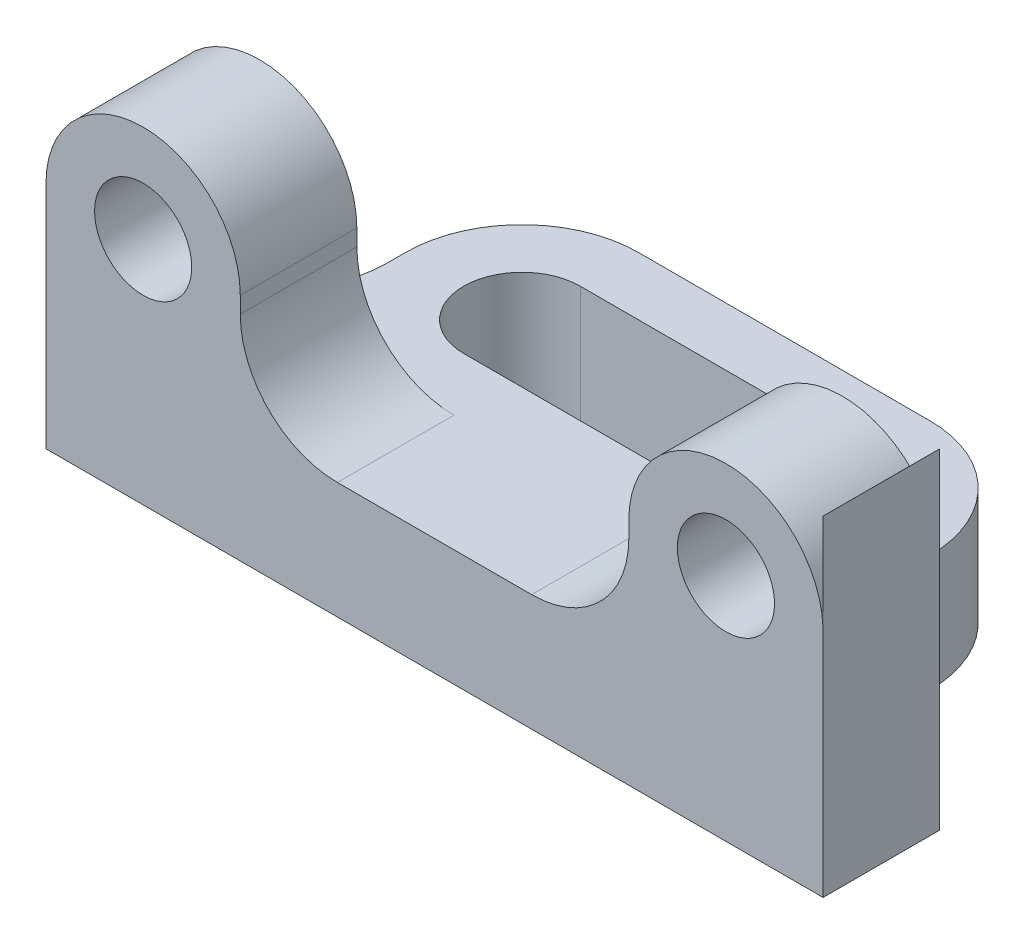
ISO-10303-21;
HEADER;
FILE_DESCRIPTION(('STEP AP214'),'2;1');
FILE_NAME('part.step','',(''),(''),'','','');
FILE_SCHEMA(('AUTOMOTIVE_DESIGN { 1 0 10303 214 1 1 1 1 }'));
ENDSEC;
DATA;
#1=APPLICATION_CONTEXT('core data for automotive mechanical design processes');
#2=APPLICATION_PROTOCOL_DEFINITION('international standard','automotive_design',2000,#1);
#3=PRODUCT_CONTEXT('',#1,'mechanical');
#4=PRODUCT('Part','Part','',(#3));
#5=PRODUCT_RELATED_PRODUCT_CATEGORY('part','',(#4));
#6=PRODUCT_DEFINITION_FORMATION('','',#4);
#7=PRODUCT_DEFINITION_CONTEXT('part definition',#1,'design');
#8=PRODUCT_DEFINITION('design','',#6,#7);
#9=PRODUCT_DEFINITION_SHAPE('','',#8);
#10=(LENGTH_UNIT() NAMED_UNIT(*) SI_UNIT(.MILLI.,.METRE.));
#11=(NAMED_UNIT(*) PLANE_ANGLE_UNIT() SI_UNIT($,.RADIAN.));
#12=(NAMED_UNIT(*) SI_UNIT($,.STERADIAN.) SOLID_ANGLE_UNIT());
#13=UNCERTAINTY_MEASURE_WITH_UNIT(LENGTH_MEASURE(1.E-05),#10,'distance_accuracy_value','');
#14=(GEOMETRIC_REPRESENTATION_CONTEXT(3) GLOBAL_UNCERTAINTY_ASSIGNED_CONTEXT((#13)) GLOBAL_UNIT_ASSIGNED_CONTEXT((#10,
#11,#12)) REPRESENTATION_CONTEXT('',''));
#15=CARTESIAN_POINT('',(0.,0.,0.));
#16=DIRECTION('',(0.,0.,1.));
#17=DIRECTION('',(1.,0.,0.));
#18=AXIS2_PLACEMENT_3D('',#15,#16,#17);
#19=CARTESIAN_POINT('',(0.,6.,0.));
#20=DIRECTION('',(0.,0.,-1.));
#21=DIRECTION('',(-1.,0.,0.));
#22=AXIS2_PLACEMENT_3D('',#19,#20,#21);
#23=PLANE('',#22);
#24=CARTESIAN_POINT('',(35.,11.844225053494,0.));
#25=DIRECTION('',(0.,0.,-1.));
#26=DIRECTION('',(-1.,0.,0.));
#27=AXIS2_PLACEMENT_3D('',#24,#25,#26);
#28=CIRCLE('',#27,2.5);
#29=CARTESIAN_POINT('',(32.5,11.844225053494,0.));
#30=VERTEX_POINT('',#29);
#31=EDGE_CURVE('E499',#30,#30,#28,.T.);
#32=ORIENTED_EDGE('',*,*,#31,.T.);
#33=EDGE_LOOP('',(#32));
#34=FACE_BOUND('',#33,.T.);
#35=CARTESIAN_POINT('',(5.,11.844225053494,0.));
#36=DIRECTION('',(0.,0.,-1.));
#37=DIRECTION('',(-1.,0.,0.));
#38=AXIS2_PLACEMENT_3D('',#35,#36,#37);
#39=CIRCLE('',#38,2.5);
#40=CARTESIAN_POINT('',(2.5,11.844225053494,0.));
#41=VERTEX_POINT('',#40);
#42=EDGE_CURVE('E505',#41,#41,#39,.T.);
#43=ORIENTED_EDGE('',*,*,#42,.T.);
#44=EDGE_LOOP('',(#43));
#45=FACE_BOUND('',#44,.T.);
#46=CARTESIAN_POINT('',(35.,11.844225053494,0.));
#47=DIRECTION('',(0.,0.,-1.));
#48=DIRECTION('',(-1.,0.,0.));
#49=AXIS2_PLACEMENT_3D('',#46,#47,#48);
#50=CIRCLE('',#49,5.);
#51=CARTESIAN_POINT('',(30.,11.844225053494,0.));
#52=VERTEX_POINT('',#51);
#53=CARTESIAN_POINT('',(39.9945012234225,12.0786552760139,0.));
#54=VERTEX_POINT('',#53);
#55=EDGE_CURVE('E467',#52,#54,#50,.T.);
#56=ORIENTED_EDGE('',*,*,#55,.F.);
#57=DIRECTION('',(0.,-1.,0.));
#58=VECTOR('',#57,1.);
#59=CARTESIAN_POINT('',(30.,17.,0.));
#60=LINE('',#59,#58);
#61=CARTESIAN_POINT('',(30.,11.,0.));
#62=VERTEX_POINT('',#61);
#63=EDGE_CURVE('E209',#52,#62,#60,.T.);
#64=ORIENTED_EDGE('',*,*,#63,.T.);
#65=CARTESIAN_POINT('',(25.,11.,0.));
#66=DIRECTION('',(0.,0.,-1.));
#67=DIRECTION('',(-1.,0.,0.));
#68=AXIS2_PLACEMENT_3D('',#65,#66,#67);
#69=CIRCLE('',#68,5.);
#70=CARTESIAN_POINT('',(25.,6.,0.));
#71=VERTEX_POINT('',#70);
#72=EDGE_CURVE('E47',#62,#71,#69,.T.);
#73=ORIENTED_EDGE('',*,*,#72,.T.);
#74=DIRECTION('',(1.,0.,0.));
#75=VECTOR('',#74,1.);
#76=CARTESIAN_POINT('',(0.,6.,0.));
#77=LINE('',#76,#75);
#78=CARTESIAN_POINT('',(15.,6.,0.));
#79=VERTEX_POINT('',#78);
#80=EDGE_CURVE('E259',#79,#71,#77,.T.);
#81=ORIENTED_EDGE('',*,*,#80,.F.);
#82=CARTESIAN_POINT('',(15.,11.,0.));
#83=DIRECTION('',(0.,0.,-1.));
#84=DIRECTION('',(-1.,0.,0.));
#85=AXIS2_PLACEMENT_3D('',#82,#83,#84);
#86=CIRCLE('',#85,5.);
#87=CARTESIAN_POINT('',(10.,11.,0.));
#88=VERTEX_POINT('',#87);
#89=EDGE_CURVE('E326',#79,#88,#86,.T.);
#90=ORIENTED_EDGE('',*,*,#89,.T.);
#91=DIRECTION('',(0.,-1.,0.));
#92=VECTOR('',#91,1.);
#93=CARTESIAN_POINT('',(10.,17.,0.));
#94=LINE('',#93,#92);
#95=CARTESIAN_POINT('',(10.,11.844225053494,0.));
#96=VERTEX_POINT('',#95);
#97=EDGE_CURVE('E493',#96,#88,#94,.T.);
#98=ORIENTED_EDGE('',*,*,#97,.F.);
#99=CARTESIAN_POINT('',(5.,11.844225053494,0.));
#100=DIRECTION('',(0.,0.,-1.));
#101=DIRECTION('',(-1.,0.,0.));
#102=AXIS2_PLACEMENT_3D('',#99,#100,#101);
#103=CIRCLE('',#102,5.);
#104=CARTESIAN_POINT('',(0.,11.844225053494,0.));
#105=VERTEX_POINT('',#104);
#106=EDGE_CURVE('E508',#105,#96,#103,.T.);
#107=ORIENTED_EDGE('',*,*,#106,.F.);
#108=DIRECTION('',(0.,-1.,0.));
#109=VECTOR('',#108,1.);
#110=CARTESIAN_POINT('',(0.,17.,0.));
#111=LINE('',#110,#109);
#112=CARTESIAN_POINT('',(0.,0.,0.));
#113=VERTEX_POINT('',#112);
#114=EDGE_CURVE('E487',#105,#113,#111,.T.);
#115=ORIENTED_EDGE('',*,*,#114,.T.);
#116=DIRECTION('',(1.,0.,0.));
#117=VECTOR('',#116,1.);
#118=CARTESIAN_POINT('',(0.,0.,0.));
#119=LINE('',#118,#117);
#120=CARTESIAN_POINT('',(40.,0.,0.));
#121=VERTEX_POINT('',#120);
#122=EDGE_CURVE('E227',#113,#121,#119,.T.);
#123=ORIENTED_EDGE('',*,*,#122,.T.);
#124=DIRECTION('',(0.,-1.,0.));
#125=VECTOR('',#124,1.);
#126=CARTESIAN_POINT('',(40.,17.,0.));
#127=LINE('',#126,#125);
#128=CARTESIAN_POINT('',(40.,17.,0.));
#129=VERTEX_POINT('',#128);
#130=EDGE_CURVE('E216',#129,#121,#127,.T.);
#131=ORIENTED_EDGE('',*,*,#130,.F.);
#132=DIRECTION('',(0.00111733143143493,0.999999375785041,0.));
#133=VECTOR('',#132,1.);
#134=CARTESIAN_POINT('',(39.9876594247451,5.95532050336561,0.));
#135=LINE('',#134,#133);
#136=EDGE_CURVE('E464',#54,#129,#135,.T.);
#137=ORIENTED_EDGE('',*,*,#136,.F.);
#138=EDGE_LOOP('',(#56,#64,#73,#81,#90,#98,#107,#115,#123,#131,#137));
#139=FACE_BOUND('',#138,.T.);
#140=ADVANCED_FACE('F41',(#34,#45,#139),#23,.F.);
#141=CARTESIAN_POINT('',(0.,17.,-6.));
#142=DIRECTION('',(0.,0.,1.));
#143=DIRECTION('',(1.,0.,0.));
#144=AXIS2_PLACEMENT_3D('',#141,#142,#143);
#145=PLANE('',#144);
#146=CARTESIAN_POINT('',(35.,11.844225053494,-6.));
#147=DIRECTION('',(0.,0.,-1.));
#148=DIRECTION('',(-1.,0.,0.));
#149=AXIS2_PLACEMENT_3D('',#146,#147,#148);
#150=CIRCLE('',#149,2.5);
#151=CARTESIAN_POINT('',(32.5,11.844225053494,-6.));
#152=VERTEX_POINT('',#151);
#153=EDGE_CURVE('E504',#152,#152,#150,.T.);
#154=ORIENTED_EDGE('',*,*,#153,.F.);
#155=EDGE_LOOP('',(#154));
#156=FACE_BOUND('',#155,.T.);
#157=CARTESIAN_POINT('',(35.,11.844225053494,-6.));
#158=DIRECTION('',(0.,0.,-1.));
#159=DIRECTION('',(-1.,0.,0.));
#160=AXIS2_PLACEMENT_3D('',#157,#158,#159);
#161=CIRCLE('',#160,5.);
#162=CARTESIAN_POINT('',(30.,11.844225053494,-6.));
#163=VERTEX_POINT('',#162);
#164=CARTESIAN_POINT('',(39.9945012234225,12.0786552760139,-5.99999999999999));
#165=VERTEX_POINT('',#164);
#166=EDGE_CURVE('E197',#163,#165,#161,.T.);
#167=ORIENTED_EDGE('',*,*,#166,.T.);
#168=DIRECTION('',(0.00111733143143494,0.999999375785041,0.));
#169=VECTOR('',#168,1.);
#170=CARTESIAN_POINT('',(39.9809554403412,-0.0446720060572272,-5.99999999999999));
#171=LINE('',#170,#169);
#172=CARTESIAN_POINT('',(40.,17.,-5.99999999999999));
#173=VERTEX_POINT('',#172);
#174=EDGE_CURVE('E203',#165,#173,#171,.T.);
#175=ORIENTED_EDGE('',*,*,#174,.T.);
#176=DIRECTION('',(0.,-1.,0.));
#177=VECTOR('',#176,1.);
#178=CARTESIAN_POINT('',(40.,17.,-6.));
#179=LINE('',#178,#177);
#180=CARTESIAN_POINT('',(40.,0.,-6.));
#181=VERTEX_POINT('',#180);
#182=EDGE_CURVE('E472',#173,#181,#179,.T.);
#183=ORIENTED_EDGE('',*,*,#182,.T.);
#184=DIRECTION('',(-1.,0.,0.));
#185=VECTOR('',#184,1.);
#186=CARTESIAN_POINT('',(0.,0.,-6.));
#187=LINE('',#186,#185);
#188=CARTESIAN_POINT('',(38.5,0.,-5.99999999999999));
#189=VERTEX_POINT('',#188);
#190=EDGE_CURVE('E479',#181,#189,#187,.T.);
#191=ORIENTED_EDGE('',*,*,#190,.T.);
#192=DIRECTION('',(0.,-1.,0.));
#193=VECTOR('',#192,1.);
#194=CARTESIAN_POINT('',(38.5,6.,-5.99999999999999));
#195=LINE('',#194,#193);
#196=CARTESIAN_POINT('',(38.5,6.,-5.99999999999999));
#197=VERTEX_POINT('',#196);
#198=EDGE_CURVE('E307',#197,#189,#195,.T.);
#199=ORIENTED_EDGE('',*,*,#198,.F.);
#200=DIRECTION('',(-1.,0.,0.));
#201=VECTOR('',#200,1.);
#202=CARTESIAN_POINT('',(0.,6.,-6.));
#203=LINE('',#202,#201);
#204=CARTESIAN_POINT('',(25.,6.,-6.));
#205=VERTEX_POINT('',#204);
#206=EDGE_CURVE('E232',#197,#205,#203,.T.);
#207=ORIENTED_EDGE('',*,*,#206,.T.);
#208=CARTESIAN_POINT('',(25.,11.,-6.));
#209=DIRECTION('',(0.,0.,1.));
#210=DIRECTION('',(1.,0.,0.));
#211=AXIS2_PLACEMENT_3D('',#208,#209,#210);
#212=CIRCLE('',#211,5.);
#213=CARTESIAN_POINT('',(30.,11.,-6.));
#214=VERTEX_POINT('',#213);
#215=EDGE_CURVE('E11',#205,#214,#212,.T.);
#216=ORIENTED_EDGE('',*,*,#215,.T.);
#217=DIRECTION('',(0.,-1.,0.));
#218=VECTOR('',#217,1.);
#219=CARTESIAN_POINT('',(30.,17.,-6.));
#220=LINE('',#219,#218);
#221=EDGE_CURVE('E61',#163,#214,#220,.T.);
#222=ORIENTED_EDGE('',*,*,#221,.F.);
#223=EDGE_LOOP('',(#167,#175,#183,#191,#199,#207,#216,#222));
#224=FACE_BOUND('',#223,.T.);
#225=ADVANCED_FACE('F212',(#156,#224),#145,.F.);
#226=CARTESIAN_POINT('',(0.,17.,-5.99999999999999));
#227=DIRECTION('',(0.,0.,-1.));
#228=DIRECTION('',(-1.,0.,0.));
#229=AXIS2_PLACEMENT_3D('',#226,#227,#228);
#230=PLANE('',#229);
#231=CARTESIAN_POINT('',(5.,11.844225053494,-6.));
#232=DIRECTION('',(0.,0.,-1.));
#233=DIRECTION('',(-1.,0.,0.));
#234=AXIS2_PLACEMENT_3D('',#231,#232,#233);
#235=CIRCLE('',#234,2.5);
#236=CARTESIAN_POINT('',(2.5,11.844225053494,-6.));
#237=VERTEX_POINT('',#236);
#238=EDGE_CURVE('E506',#237,#237,#235,.T.);
#239=ORIENTED_EDGE('',*,*,#238,.F.);
#240=EDGE_LOOP('',(#239));
#241=FACE_BOUND('',#240,.T.);
#242=DIRECTION('',(0.,-1.,0.));
#243=VECTOR('',#242,1.);
#244=CARTESIAN_POINT('',(0.,17.,-5.99999999999999));
#245=LINE('',#244,#243);
#246=CARTESIAN_POINT('',(0.,11.844225053494,-5.99999999999999));
#247=VERTEX_POINT('',#246);
#248=CARTESIAN_POINT('',(0.,0.,-5.99999999999999));
#249=VERTEX_POINT('',#248);
#250=EDGE_CURVE('E481',#247,#249,#245,.T.);
#251=ORIENTED_EDGE('',*,*,#250,.F.);
#252=CARTESIAN_POINT('',(5.,11.844225053494,-6.));
#253=DIRECTION('',(0.,0.,-1.));
#254=DIRECTION('',(-1.,0.,0.));
#255=AXIS2_PLACEMENT_3D('',#252,#253,#254);
#256=CIRCLE('',#255,5.);
#257=CARTESIAN_POINT('',(10.,11.844225053494,-6.));
#258=VERTEX_POINT('',#257);
#259=EDGE_CURVE('E57',#247,#258,#256,.T.);
#260=ORIENTED_EDGE('',*,*,#259,.T.);
#261=DIRECTION('',(0.,-1.,0.));
#262=VECTOR('',#261,1.);
#263=CARTESIAN_POINT('',(10.,17.,-6.));
#264=LINE('',#263,#262);
#265=CARTESIAN_POINT('',(10.,11.,-6.));
#266=VERTEX_POINT('',#265);
#267=EDGE_CURVE('E482',#258,#266,#264,.T.);
#268=ORIENTED_EDGE('',*,*,#267,.T.);
#269=CARTESIAN_POINT('',(15.,11.,-6.));
#270=DIRECTION('',(0.,0.,-1.));
#271=DIRECTION('',(-1.,0.,0.));
#272=AXIS2_PLACEMENT_3D('',#269,#270,#271);
#273=CIRCLE('',#272,5.);
#274=CARTESIAN_POINT('',(15.,6.,-6.));
#275=VERTEX_POINT('',#274);
#276=EDGE_CURVE('E334',#266,#275,#273,.F.);
#277=ORIENTED_EDGE('',*,*,#276,.T.);
#278=DIRECTION('',(1.,0.,0.));
#279=VECTOR('',#278,1.);
#280=CARTESIAN_POINT('',(0.,6.,-5.99999999999999));
#281=LINE('',#280,#279);
#282=CARTESIAN_POINT('',(1.49999999999996,6.,-5.99999999999999));
#283=VERTEX_POINT('',#282);
#284=EDGE_CURVE('E257',#283,#275,#281,.T.);
#285=ORIENTED_EDGE('',*,*,#284,.F.);
#286=DIRECTION('',(0.,-1.,0.));
#287=VECTOR('',#286,1.);
#288=CARTESIAN_POINT('',(1.49999999999996,6.,-5.99999999999999));
#289=LINE('',#288,#287);
#290=CARTESIAN_POINT('',(1.49999999999996,0.,-5.99999999999999));
#291=VERTEX_POINT('',#290);
#292=EDGE_CURVE('E292',#283,#291,#289,.T.);
#293=ORIENTED_EDGE('',*,*,#292,.T.);
#294=DIRECTION('',(1.,0.,0.));
#295=VECTOR('',#294,1.);
#296=CARTESIAN_POINT('',(0.,0.,-5.99999999999999));
#297=LINE('',#296,#295);
#298=EDGE_CURVE('E500',#249,#291,#297,.T.);
#299=ORIENTED_EDGE('',*,*,#298,.F.);
#300=EDGE_LOOP('',(#251,#260,#268,#277,#285,#293,#299));
#301=FACE_BOUND('',#300,.T.);
#302=ADVANCED_FACE('F365',(#241,#301),#230,.T.);
#303=CARTESIAN_POINT('',(38.5,6.,-11.));
#304=DIRECTION('',(0.,-1.,0.));
#305=DIRECTION('',(0.,0.,-1.));
#306=AXIS2_PLACEMENT_3D('',#303,#304,#305);
#307=CYLINDRICAL_SURFACE('',#306,5.);
#308=CARTESIAN_POINT('',(38.5,0.,-11.));
#309=DIRECTION('',(0.,1.,0.));
#310=DIRECTION('',(0.,0.,1.));
#311=AXIS2_PLACEMENT_3D('',#308,#309,#310);
#312=CIRCLE('',#311,5.);
#313=CARTESIAN_POINT('',(33.5,0.,-11.));
#314=VERTEX_POINT('',#313);
#315=EDGE_CURVE('E268',#189,#314,#312,.F.);
#316=ORIENTED_EDGE('',*,*,#315,.T.);
#317=DIRECTION('',(0.,-1.,0.));
#318=VECTOR('',#317,1.);
#319=CARTESIAN_POINT('',(33.5,6.,-11.));
#320=LINE('',#319,#318);
#321=CARTESIAN_POINT('',(33.5,6.,-11.));
#322=VERTEX_POINT('',#321);
#323=EDGE_CURVE('E306',#322,#314,#320,.T.);
#324=ORIENTED_EDGE('',*,*,#323,.F.);
#325=CARTESIAN_POINT('',(38.5,6.,-11.));
#326=DIRECTION('',(0.,1.,0.));
#327=DIRECTION('',(0.,0.,1.));
#328=AXIS2_PLACEMENT_3D('',#325,#326,#327);
#329=CIRCLE('',#328,5.);
#330=EDGE_CURVE('E240',#197,#322,#329,.F.);
#331=ORIENTED_EDGE('',*,*,#330,.F.);
#332=ORIENTED_EDGE('',*,*,#198,.T.);
#333=EDGE_LOOP('',(#316,#324,#331,#332));
#334=FACE_BOUND('',#333,.T.);
#335=ADVANCED_FACE('F393',(#334),#307,.F.);
#336=CARTESIAN_POINT('',(33.5,6.,0.));
#337=DIRECTION('',(-1.,0.,0.));
#338=DIRECTION('',(0.,0.,1.));
#339=AXIS2_PLACEMENT_3D('',#336,#337,#338);
#340=PLANE('',#339);
#341=DIRECTION('',(0.,0.,-1.));
#342=VECTOR('',#341,1.);
#343=CARTESIAN_POINT('',(33.5,0.,0.));
#344=LINE('',#343,#342);
#345=CARTESIAN_POINT('',(33.5,0.,-12.));
#346=VERTEX_POINT('',#345);
#347=EDGE_CURVE('E271',#314,#346,#344,.T.);
#348=ORIENTED_EDGE('',*,*,#347,.T.);
#349=DIRECTION('',(0.,-1.,0.));
#350=VECTOR('',#349,1.);
#351=CARTESIAN_POINT('',(33.5,6.,-12.));
#352=LINE('',#351,#350);
#353=CARTESIAN_POINT('',(33.5,6.,-12.));
#354=VERTEX_POINT('',#353);
#355=EDGE_CURVE('E302',#354,#346,#352,.T.);
#356=ORIENTED_EDGE('',*,*,#355,.F.);
#357=DIRECTION('',(0.,0.,-1.));
#358=VECTOR('',#357,1.);
#359=CARTESIAN_POINT('',(33.5,6.,0.));
#360=LINE('',#359,#358);
#361=EDGE_CURVE('E239',#322,#354,#360,.T.);
#362=ORIENTED_EDGE('',*,*,#361,.F.);
#363=ORIENTED_EDGE('',*,*,#323,.T.);
#364=EDGE_LOOP('',(#348,#356,#362,#363));
#365=FACE_BOUND('',#364,.T.);
#366=ADVANCED_FACE('F392',(#365),#340,.F.);
#367=CARTESIAN_POINT('',(27.5,6.,-12.));
#368=DIRECTION('',(0.,-1.,0.));
#369=DIRECTION('',(0.,0.,-1.));
#370=AXIS2_PLACEMENT_3D('',#367,#368,#369);
#371=CYLINDRICAL_SURFACE('',#370,6.);
#372=CARTESIAN_POINT('',(27.5,0.,-12.));
#373=DIRECTION('',(0.,1.,0.));
#374=DIRECTION('',(0.,0.,1.));
#375=AXIS2_PLACEMENT_3D('',#372,#373,#374);
#376=CIRCLE('',#375,6.);
#377=CARTESIAN_POINT('',(27.5,0.,-18.));
#378=VERTEX_POINT('',#377);
#379=EDGE_CURVE('E277',#378,#346,#376,.F.);
#380=ORIENTED_EDGE('',*,*,#379,.F.);
#381=DIRECTION('',(0.,-1.,0.));
#382=VECTOR('',#381,1.);
#383=CARTESIAN_POINT('',(27.5,6.,-18.));
#384=LINE('',#383,#382);
#385=CARTESIAN_POINT('',(27.5,6.,-18.));
#386=VERTEX_POINT('',#385);
#387=EDGE_CURVE('E305',#386,#378,#384,.T.);
#388=ORIENTED_EDGE('',*,*,#387,.F.);
#389=CARTESIAN_POINT('',(27.5,6.,-12.));
#390=DIRECTION('',(0.,1.,0.));
#391=DIRECTION('',(0.,0.,1.));
#392=AXIS2_PLACEMENT_3D('',#389,#390,#391);
#393=CIRCLE('',#392,6.);
#394=EDGE_CURVE('E245',#386,#354,#393,.F.);
#395=ORIENTED_EDGE('',*,*,#394,.T.);
#396=ORIENTED_EDGE('',*,*,#355,.T.);
#397=EDGE_LOOP('',(#380,#388,#395,#396));
#398=FACE_BOUND('',#397,.T.);
#399=ADVANCED_FACE('F390',(#398),#371,.T.);
#400=CARTESIAN_POINT('',(0.,6.,-18.));
#401=DIRECTION('',(0.,0.,-1.));
#402=DIRECTION('',(-1.,0.,0.));
#403=AXIS2_PLACEMENT_3D('',#400,#401,#402);
#404=PLANE('',#403);
#405=DIRECTION('',(1.,0.,0.));
#406=VECTOR('',#405,1.);
#407=CARTESIAN_POINT('',(0.,0.,-18.));
#408=LINE('',#407,#406);
#409=CARTESIAN_POINT('',(12.5,0.,-18.));
#410=VERTEX_POINT('',#409);
#411=EDGE_CURVE('E276',#410,#378,#408,.T.);
#412=ORIENTED_EDGE('',*,*,#411,.F.);
#413=DIRECTION('',(0.,-1.,0.));
#414=VECTOR('',#413,1.);
#415=CARTESIAN_POINT('',(12.5,6.,-18.));
#416=LINE('',#415,#414);
#417=CARTESIAN_POINT('',(12.5,6.,-18.));
#418=VERTEX_POINT('',#417);
#419=EDGE_CURVE('E297',#418,#410,#416,.T.);
#420=ORIENTED_EDGE('',*,*,#419,.F.);
#421=DIRECTION('',(1.,0.,0.));
#422=VECTOR('',#421,1.);
#423=CARTESIAN_POINT('',(0.,6.,-18.));
#424=LINE('',#423,#422);
#425=EDGE_CURVE('E244',#418,#386,#424,.T.);
#426=ORIENTED_EDGE('',*,*,#425,.T.);
#427=ORIENTED_EDGE('',*,*,#387,.T.);
#428=EDGE_LOOP('',(#412,#420,#426,#427));
#429=FACE_BOUND('',#428,.T.);
#430=ADVANCED_FACE('F384',(#429),#404,.T.);
#431=CARTESIAN_POINT('',(12.5,6.,-12.));
#432=DIRECTION('',(0.,-1.,0.));
#433=DIRECTION('',(0.,0.,-1.));
#434=AXIS2_PLACEMENT_3D('',#431,#432,#433);
#435=CYLINDRICAL_SURFACE('',#434,6.);
#436=CARTESIAN_POINT('',(12.5,0.,-12.));
#437=DIRECTION('',(0.,1.,0.));
#438=DIRECTION('',(0.,0.,1.));
#439=AXIS2_PLACEMENT_3D('',#436,#437,#438);
#440=CIRCLE('',#439,6.);
#441=CARTESIAN_POINT('',(6.5,0.,-12.));
#442=VERTEX_POINT('',#441);
#443=EDGE_CURVE('E284',#410,#442,#440,.T.);
#444=ORIENTED_EDGE('',*,*,#443,.T.);
#445=DIRECTION('',(0.,-1.,0.));
#446=VECTOR('',#445,1.);
#447=CARTESIAN_POINT('',(6.5,6.,-12.));
#448=LINE('',#447,#446);
#449=CARTESIAN_POINT('',(6.5,6.,-12.));
#450=VERTEX_POINT('',#449);
#451=EDGE_CURVE('E296',#450,#442,#448,.T.);
#452=ORIENTED_EDGE('',*,*,#451,.F.);
#453=CARTESIAN_POINT('',(12.5,6.,-12.));
#454=DIRECTION('',(0.,1.,0.));
#455=DIRECTION('',(0.,0.,1.));
#456=AXIS2_PLACEMENT_3D('',#453,#454,#455);
#457=CIRCLE('',#456,6.);
#458=EDGE_CURVE('E247',#418,#450,#457,.T.);
#459=ORIENTED_EDGE('',*,*,#458,.F.);
#460=ORIENTED_EDGE('',*,*,#419,.T.);
#461=EDGE_LOOP('',(#444,#452,#459,#460));
#462=FACE_BOUND('',#461,.T.);
#463=ADVANCED_FACE('F378',(#462),#435,.T.);
#464=CARTESIAN_POINT('',(6.5,6.,0.));
#465=DIRECTION('',(-1.,0.,0.));
#466=DIRECTION('',(0.,0.,1.));
#467=AXIS2_PLACEMENT_3D('',#464,#465,#466);
#468=PLANE('',#467);
#469=DIRECTION('',(0.,0.,-1.));
#470=VECTOR('',#469,1.);
#471=CARTESIAN_POINT('',(6.5,0.,0.));
#472=LINE('',#471,#470);
#473=CARTESIAN_POINT('',(6.5,0.,-11.));
#474=VERTEX_POINT('',#473);
#475=EDGE_CURVE('E283',#474,#442,#472,.T.);
#476=ORIENTED_EDGE('',*,*,#475,.F.);
#477=DIRECTION('',(0.,-1.,0.));
#478=VECTOR('',#477,1.);
#479=CARTESIAN_POINT('',(6.5,6.,-11.));
#480=LINE('',#479,#478);
#481=CARTESIAN_POINT('',(6.5,6.,-11.));
#482=VERTEX_POINT('',#481);
#483=EDGE_CURVE('E294',#482,#474,#480,.T.);
#484=ORIENTED_EDGE('',*,*,#483,.F.);
#485=DIRECTION('',(0.,0.,-1.));
#486=VECTOR('',#485,1.);
#487=CARTESIAN_POINT('',(6.5,6.,0.));
#488=LINE('',#487,#486);
#489=EDGE_CURVE('E249',#482,#450,#488,.T.);
#490=ORIENTED_EDGE('',*,*,#489,.T.);
#491=ORIENTED_EDGE('',*,*,#451,.T.);
#492=EDGE_LOOP('',(#476,#484,#490,#491));
#493=FACE_BOUND('',#492,.T.);
#494=ADVANCED_FACE('F374',(#493),#468,.T.);
#495=CARTESIAN_POINT('',(1.5,6.,-11.));
#496=DIRECTION('',(0.,-1.,0.));
#497=DIRECTION('',(0.,0.,-1.));
#498=AXIS2_PLACEMENT_3D('',#495,#496,#497);
#499=CYLINDRICAL_SURFACE('',#498,5.);
#500=CARTESIAN_POINT('',(1.5,0.,-11.));
#501=DIRECTION('',(0.,1.,0.));
#502=DIRECTION('',(0.,0.,1.));
#503=AXIS2_PLACEMENT_3D('',#500,#501,#502);
#504=CIRCLE('',#503,5.);
#505=EDGE_CURVE('E290',#291,#474,#504,.T.);
#506=ORIENTED_EDGE('',*,*,#505,.F.);
#507=ORIENTED_EDGE('',*,*,#292,.F.);
#508=CARTESIAN_POINT('',(1.5,6.,-11.));
#509=DIRECTION('',(0.,1.,0.));
#510=DIRECTION('',(0.,0.,1.));
#511=AXIS2_PLACEMENT_3D('',#508,#509,#510);
#512=CIRCLE('',#511,5.);
#513=EDGE_CURVE('E254',#283,#482,#512,.T.);
#514=ORIENTED_EDGE('',*,*,#513,.T.);
#515=ORIENTED_EDGE('',*,*,#483,.T.);
#516=EDGE_LOOP('',(#506,#507,#514,#515));
#517=FACE_BOUND('',#516,.T.);
#518=ADVANCED_FACE('F371',(#517),#499,.F.);
#519=CARTESIAN_POINT('',(27.5,6.,-12.));
#520=DIRECTION('',(0.,-1.,0.));
#521=DIRECTION('',(0.,0.,-1.));
#522=AXIS2_PLACEMENT_3D('',#519,#520,#521);
#523=CYLINDRICAL_SURFACE('',#522,3.);
#524=CARTESIAN_POINT('',(27.5,0.,-12.));
#525=DIRECTION('',(0.,1.,0.));
#526=DIRECTION('',(0.,0.,1.));
#527=AXIS2_PLACEMENT_3D('',#524,#525,#526);
#528=CIRCLE('',#527,3.);
#529=CARTESIAN_POINT('',(27.5,0.,-9.));
#530=VERTEX_POINT('',#529);
#531=CARTESIAN_POINT('',(27.5,0.,-15.));
#532=VERTEX_POINT('',#531);
#533=EDGE_CURVE('E211',#530,#532,#528,.T.);
#534=ORIENTED_EDGE('',*,*,#533,.F.);
#535=DIRECTION('',(0.,-1.,0.));
#536=VECTOR('',#535,1.);
#537=CARTESIAN_POINT('',(27.5,6.,-9.));
#538=LINE('',#537,#536);
#539=CARTESIAN_POINT('',(27.5,6.,-9.));
#540=VERTEX_POINT('',#539);
#541=EDGE_CURVE('E298',#540,#530,#538,.T.);
#542=ORIENTED_EDGE('',*,*,#541,.F.);
#543=CARTESIAN_POINT('',(27.5,6.,-12.));
#544=DIRECTION('',(0.,1.,0.));
#545=DIRECTION('',(0.,0.,1.));
#546=AXIS2_PLACEMENT_3D('',#543,#544,#545);
#547=CIRCLE('',#546,3.);
#548=CARTESIAN_POINT('',(27.5,6.,-15.));
#549=VERTEX_POINT('',#548);
#550=EDGE_CURVE('E225',#540,#549,#547,.T.);
#551=ORIENTED_EDGE('',*,*,#550,.T.);
#552=DIRECTION('',(0.,-1.,0.));
#553=VECTOR('',#552,1.);
#554=CARTESIAN_POINT('',(27.5,6.,-15.));
#555=LINE('',#554,#553);
#556=EDGE_CURVE('E258',#549,#532,#555,.T.);
#557=ORIENTED_EDGE('',*,*,#556,.T.);
#558=EDGE_LOOP('',(#534,#542,#551,#557));
#559=FACE_BOUND('',#558,.T.);
#560=ADVANCED_FACE('F372',(#559),#523,.F.);
#561=CARTESIAN_POINT('',(0.,6.,-9.));
#562=DIRECTION('',(0.,0.,-1.));
#563=DIRECTION('',(-1.,0.,0.));
#564=AXIS2_PLACEMENT_3D('',#561,#562,#563);
#565=PLANE('',#564);
#566=DIRECTION('',(1.,0.,0.));
#567=VECTOR('',#566,1.);
#568=CARTESIAN_POINT('',(0.,0.,-9.));
#569=LINE('',#568,#567);
#570=CARTESIAN_POINT('',(12.5,0.,-9.));
#571=VERTEX_POINT('',#570);
#572=EDGE_CURVE('E219',#571,#530,#569,.T.);
#573=ORIENTED_EDGE('',*,*,#572,.F.);
#574=DIRECTION('',(0.,-1.,0.));
#575=VECTOR('',#574,1.);
#576=CARTESIAN_POINT('',(12.5,6.,-9.));
#577=LINE('',#576,#575);
#578=CARTESIAN_POINT('',(12.5,6.,-9.));
#579=VERTEX_POINT('',#578);
#580=EDGE_CURVE('E317',#579,#571,#577,.T.);
#581=ORIENTED_EDGE('',*,*,#580,.F.);
#582=DIRECTION('',(1.,0.,0.));
#583=VECTOR('',#582,1.);
#584=CARTESIAN_POINT('',(0.,6.,-9.));
#585=LINE('',#584,#583);
#586=EDGE_CURVE('E228',#579,#540,#585,.T.);
#587=ORIENTED_EDGE('',*,*,#586,.T.);
#588=ORIENTED_EDGE('',*,*,#541,.T.);
#589=EDGE_LOOP('',(#573,#581,#587,#588));
#590=FACE_BOUND('',#589,.T.);
#591=ADVANCED_FACE('F410',(#590),#565,.T.);
#592=CARTESIAN_POINT('',(12.5,6.,-12.));
#593=DIRECTION('',(0.,-1.,0.));
#594=DIRECTION('',(0.,0.,-1.));
#595=AXIS2_PLACEMENT_3D('',#592,#593,#594);
#596=CYLINDRICAL_SURFACE('',#595,3.);
#597=CARTESIAN_POINT('',(12.5,0.,-12.));
#598=DIRECTION('',(0.,1.,0.));
#599=DIRECTION('',(0.,0.,1.));
#600=AXIS2_PLACEMENT_3D('',#597,#598,#599);
#601=CIRCLE('',#600,3.);
#602=CARTESIAN_POINT('',(12.5,0.,-15.));
#603=VERTEX_POINT('',#602);
#604=EDGE_CURVE('E261',#603,#571,#601,.T.);
#605=ORIENTED_EDGE('',*,*,#604,.F.);
#606=DIRECTION('',(0.,-1.,0.));
#607=VECTOR('',#606,1.);
#608=CARTESIAN_POINT('',(12.5,6.,-15.));
#609=LINE('',#608,#607);
#610=CARTESIAN_POINT('',(12.5,6.,-15.));
#611=VERTEX_POINT('',#610);
#612=EDGE_CURVE('E313',#611,#603,#609,.T.);
#613=ORIENTED_EDGE('',*,*,#612,.F.);
#614=CARTESIAN_POINT('',(12.5,6.,-12.));
#615=DIRECTION('',(0.,1.,0.));
#616=DIRECTION('',(0.,0.,1.));
#617=AXIS2_PLACEMENT_3D('',#614,#615,#616);
#618=CIRCLE('',#617,3.);
#619=EDGE_CURVE('E229',#611,#579,#618,.T.);
#620=ORIENTED_EDGE('',*,*,#619,.T.);
#621=ORIENTED_EDGE('',*,*,#580,.T.);
#622=EDGE_LOOP('',(#605,#613,#620,#621));
#623=FACE_BOUND('',#622,.T.);
#624=ADVANCED_FACE('F401',(#623),#596,.F.);
#625=CARTESIAN_POINT('',(0.,6.,-15.));
#626=DIRECTION('',(0.,0.,-1.));
#627=DIRECTION('',(-1.,0.,0.));
#628=AXIS2_PLACEMENT_3D('',#625,#626,#627);
#629=PLANE('',#628);
#630=DIRECTION('',(1.,0.,0.));
#631=VECTOR('',#630,1.);
#632=CARTESIAN_POINT('',(0.,0.,-15.));
#633=LINE('',#632,#631);
#634=EDGE_CURVE('E269',#603,#532,#633,.T.);
#635=ORIENTED_EDGE('',*,*,#634,.T.);
#636=ORIENTED_EDGE('',*,*,#556,.F.);
#637=DIRECTION('',(1.,0.,0.));
#638=VECTOR('',#637,1.);
#639=CARTESIAN_POINT('',(0.,6.,-15.));
#640=LINE('',#639,#638);
#641=EDGE_CURVE('E231',#611,#549,#640,.T.);
#642=ORIENTED_EDGE('',*,*,#641,.F.);
#643=ORIENTED_EDGE('',*,*,#612,.T.);
#644=EDGE_LOOP('',(#635,#636,#642,#643));
#645=FACE_BOUND('',#644,.T.);
#646=ADVANCED_FACE('F398',(#645),#629,.F.);
#647=CARTESIAN_POINT('',(0.,6.,0.));
#648=DIRECTION('',(0.,1.,0.));
#649=DIRECTION('',(0.,0.,1.));
#650=AXIS2_PLACEMENT_3D('',#647,#648,#649);
#651=PLANE('',#650);
#652=ORIENTED_EDGE('',*,*,#550,.F.);
#653=ORIENTED_EDGE('',*,*,#586,.F.);
#654=ORIENTED_EDGE('',*,*,#619,.F.);
#655=ORIENTED_EDGE('',*,*,#641,.T.);
#656=EDGE_LOOP('',(#652,#653,#654,#655));
#657=FACE_BOUND('',#656,.T.);
#658=ORIENTED_EDGE('',*,*,#284,.T.);
#659=DIRECTION('',(0.,0.,1.));
#660=VECTOR('',#659,1.);
#661=CARTESIAN_POINT('',(15.,6.,0.));
#662=LINE('',#661,#660);
#663=EDGE_CURVE('E322',#275,#79,#662,.T.);
#664=ORIENTED_EDGE('',*,*,#663,.T.);
#665=ORIENTED_EDGE('',*,*,#80,.T.);
#666=DIRECTION('',(0.,0.,1.));
#667=VECTOR('',#666,1.);
#668=CARTESIAN_POINT('',(25.,6.,0.));
#669=LINE('',#668,#667);
#670=EDGE_CURVE('E315',#71,#205,#669,.F.);
#671=ORIENTED_EDGE('',*,*,#670,.T.);
#672=ORIENTED_EDGE('',*,*,#206,.F.);
#673=ORIENTED_EDGE('',*,*,#330,.T.);
#674=ORIENTED_EDGE('',*,*,#361,.T.);
#675=ORIENTED_EDGE('',*,*,#394,.F.);
#676=ORIENTED_EDGE('',*,*,#425,.F.);
#677=ORIENTED_EDGE('',*,*,#458,.T.);
#678=ORIENTED_EDGE('',*,*,#489,.F.);
#679=ORIENTED_EDGE('',*,*,#513,.F.);
#680=EDGE_LOOP('',(#658,#664,#665,#671,#672,#673,#674,#675,#676,#677,#678,#679));
#681=FACE_BOUND('',#680,.T.);
#682=ADVANCED_FACE('F338',(#657,#681),#651,.T.);
#683=CARTESIAN_POINT('',(0.,0.,0.));
#684=DIRECTION('',(0.,1.,0.));
#685=DIRECTION('',(0.,0.,1.));
#686=AXIS2_PLACEMENT_3D('',#683,#684,#685);
#687=PLANE('',#686);
#688=ORIENTED_EDGE('',*,*,#122,.F.);
#689=DIRECTION('',(0.,0.,1.));
#690=VECTOR('',#689,1.);
#691=CARTESIAN_POINT('',(0.,0.,0.));
#692=LINE('',#691,#690);
#693=EDGE_CURVE('E492',#249,#113,#692,.T.);
#694=ORIENTED_EDGE('',*,*,#693,.F.);
#695=ORIENTED_EDGE('',*,*,#298,.T.);
#696=ORIENTED_EDGE('',*,*,#505,.T.);
#697=ORIENTED_EDGE('',*,*,#475,.T.);
#698=ORIENTED_EDGE('',*,*,#443,.F.);
#699=ORIENTED_EDGE('',*,*,#411,.T.);
#700=ORIENTED_EDGE('',*,*,#379,.T.);
#701=ORIENTED_EDGE('',*,*,#347,.F.);
#702=ORIENTED_EDGE('',*,*,#315,.F.);
#703=ORIENTED_EDGE('',*,*,#190,.F.);
#704=DIRECTION('',(0.,0.,-1.));
#705=VECTOR('',#704,1.);
#706=CARTESIAN_POINT('',(40.,0.,0.));
#707=LINE('',#706,#705);
#708=EDGE_CURVE('E471',#121,#181,#707,.T.);
#709=ORIENTED_EDGE('',*,*,#708,.F.);
#710=EDGE_LOOP('',(#688,#694,#695,#696,#697,#698,#699,#700,#701,#702,#703,#709));
#711=FACE_BOUND('',#710,.T.);
#712=ORIENTED_EDGE('',*,*,#533,.T.);
#713=ORIENTED_EDGE('',*,*,#634,.F.);
#714=ORIENTED_EDGE('',*,*,#604,.T.);
#715=ORIENTED_EDGE('',*,*,#572,.T.);
#716=EDGE_LOOP('',(#712,#713,#714,#715));
#717=FACE_BOUND('',#716,.T.);
#718=ADVANCED_FACE('F367',(#711,#717),#687,.F.);
#719=CARTESIAN_POINT('',(30.,17.,0.));
#720=DIRECTION('',(1.,0.,0.));
#721=DIRECTION('',(0.,0.,-1.));
#722=AXIS2_PLACEMENT_3D('',#719,#720,#721);
#723=PLANE('',#722);
#724=ORIENTED_EDGE('',*,*,#63,.F.);
#725=DIRECTION('',(0.,0.,-1.));
#726=VECTOR('',#725,1.);
#727=CARTESIAN_POINT('',(30.,11.844225053494,11.));
#728=LINE('',#727,#726);
#729=EDGE_CURVE('E200',#52,#163,#728,.T.);
#730=ORIENTED_EDGE('',*,*,#729,.T.);
#731=ORIENTED_EDGE('',*,*,#221,.T.);
#732=DIRECTION('',(0.,0.,1.));
#733=VECTOR('',#732,1.);
#734=CARTESIAN_POINT('',(30.,11.,0.));
#735=LINE('',#734,#733);
#736=EDGE_CURVE('E329',#214,#62,#735,.T.);
#737=ORIENTED_EDGE('',*,*,#736,.T.);
#738=EDGE_LOOP('',(#724,#730,#731,#737));
#739=FACE_BOUND('',#738,.T.);
#740=ADVANCED_FACE('F206',(#739),#723,.F.);
#741=CARTESIAN_POINT('',(40.,17.,0.));
#742=DIRECTION('',(-1.,0.,0.));
#743=DIRECTION('',(0.,0.,1.));
#744=AXIS2_PLACEMENT_3D('',#741,#742,#743);
#745=PLANE('',#744);
#746=ORIENTED_EDGE('',*,*,#708,.T.);
#747=ORIENTED_EDGE('',*,*,#182,.F.);
#748=DIRECTION('',(0.,0.,-1.));
#749=VECTOR('',#748,1.);
#750=CARTESIAN_POINT('',(40.,17.,0.));
#751=LINE('',#750,#749);
#752=EDGE_CURVE('E463',#129,#173,#751,.T.);
#753=ORIENTED_EDGE('',*,*,#752,.F.);
#754=ORIENTED_EDGE('',*,*,#130,.T.);
#755=EDGE_LOOP('',(#746,#747,#753,#754));
#756=FACE_BOUND('',#755,.T.);
#757=ADVANCED_FACE('F434',(#756),#745,.F.);
#758=CARTESIAN_POINT('',(10.,17.,0.));
#759=DIRECTION('',(1.,0.,0.));
#760=DIRECTION('',(0.,0.,-1.));
#761=AXIS2_PLACEMENT_3D('',#758,#759,#760);
#762=PLANE('',#761);
#763=DIRECTION('',(0.,0.,-1.));
#764=VECTOR('',#763,1.);
#765=CARTESIAN_POINT('',(10.,11.844225053494,11.));
#766=LINE('',#765,#764);
#767=EDGE_CURVE('E514',#96,#258,#766,.T.);
#768=ORIENTED_EDGE('',*,*,#767,.F.);
#769=ORIENTED_EDGE('',*,*,#97,.T.);
#770=DIRECTION('',(0.,0.,1.));
#771=VECTOR('',#770,1.);
#772=CARTESIAN_POINT('',(10.,11.,-6.));
#773=LINE('',#772,#771);
#774=EDGE_CURVE('E321',#88,#266,#773,.F.);
#775=ORIENTED_EDGE('',*,*,#774,.T.);
#776=ORIENTED_EDGE('',*,*,#267,.F.);
#777=EDGE_LOOP('',(#768,#769,#775,#776));
#778=FACE_BOUND('',#777,.T.);
#779=ADVANCED_FACE('F438',(#778),#762,.T.);
#780=CARTESIAN_POINT('',(0.,17.,0.));
#781=DIRECTION('',(1.,0.,0.));
#782=DIRECTION('',(0.,0.,-1.));
#783=AXIS2_PLACEMENT_3D('',#780,#781,#782);
#784=PLANE('',#783);
#785=ORIENTED_EDGE('',*,*,#114,.F.);
#786=DIRECTION('',(0.,0.,-1.));
#787=VECTOR('',#786,1.);
#788=CARTESIAN_POINT('',(0.,11.844225053494,11.));
#789=LINE('',#788,#787);
#790=EDGE_CURVE('E511',#105,#247,#789,.T.);
#791=ORIENTED_EDGE('',*,*,#790,.T.);
#792=ORIENTED_EDGE('',*,*,#250,.T.);
#793=ORIENTED_EDGE('',*,*,#693,.T.);
#794=EDGE_LOOP('',(#785,#791,#792,#793));
#795=FACE_BOUND('',#794,.T.);
#796=ADVANCED_FACE('F355',(#795),#784,.F.);
#797=CARTESIAN_POINT('',(15.,11.,0.));
#798=DIRECTION('',(0.,0.,-1.));
#799=DIRECTION('',(-1.,0.,0.));
#800=AXIS2_PLACEMENT_3D('',#797,#798,#799);
#801=CYLINDRICAL_SURFACE('',#800,5.);
#802=ORIENTED_EDGE('',*,*,#276,.F.);
#803=ORIENTED_EDGE('',*,*,#774,.F.);
#804=ORIENTED_EDGE('',*,*,#89,.F.);
#805=ORIENTED_EDGE('',*,*,#663,.F.);
#806=EDGE_LOOP('',(#802,#803,#804,#805));
#807=FACE_BOUND('',#806,.T.);
#808=ADVANCED_FACE('F343',(#807),#801,.F.);
#809=CARTESIAN_POINT('',(25.,11.,0.));
#810=DIRECTION('',(0.,0.,1.));
#811=DIRECTION('',(1.,0.,0.));
#812=AXIS2_PLACEMENT_3D('',#809,#810,#811);
#813=CYLINDRICAL_SURFACE('',#812,5.);
#814=ORIENTED_EDGE('',*,*,#215,.F.);
#815=ORIENTED_EDGE('',*,*,#670,.F.);
#816=ORIENTED_EDGE('',*,*,#72,.F.);
#817=ORIENTED_EDGE('',*,*,#736,.F.);
#818=EDGE_LOOP('',(#814,#815,#816,#817));
#819=FACE_BOUND('',#818,.T.);
#820=ADVANCED_FACE('F43',(#819),#813,.F.);
#821=CARTESIAN_POINT('',(5.,11.844225053494,11.));
#822=DIRECTION('',(0.,0.,-1.));
#823=DIRECTION('',(-1.,0.,0.));
#824=AXIS2_PLACEMENT_3D('',#821,#822,#823);
#825=CYLINDRICAL_SURFACE('',#824,2.5);
#826=ORIENTED_EDGE('',*,*,#238,.T.);
#827=EDGE_LOOP('',(#826));
#828=FACE_BOUND('',#827,.T.);
#829=ORIENTED_EDGE('',*,*,#42,.F.);
#830=EDGE_LOOP('',(#829));
#831=FACE_BOUND('',#830,.T.);
#832=ADVANCED_FACE('F341',(#828,#831),#825,.F.);
#833=CARTESIAN_POINT('',(35.,11.844225053494,11.));
#834=DIRECTION('',(0.,0.,-1.));
#835=DIRECTION('',(-1.,0.,0.));
#836=AXIS2_PLACEMENT_3D('',#833,#834,#835);
#837=CYLINDRICAL_SURFACE('',#836,2.5);
#838=ORIENTED_EDGE('',*,*,#153,.T.);
#839=EDGE_LOOP('',(#838));
#840=FACE_BOUND('',#839,.T.);
#841=ORIENTED_EDGE('',*,*,#31,.F.);
#842=EDGE_LOOP('',(#841));
#843=FACE_BOUND('',#842,.T.);
#844=ADVANCED_FACE('F348',(#840,#843),#837,.F.);
#845=CARTESIAN_POINT('',(5.,11.844225053494,11.));
#846=DIRECTION('',(0.,0.,-1.));
#847=DIRECTION('',(-1.,0.,0.));
#848=AXIS2_PLACEMENT_3D('',#845,#846,#847);
#849=CYLINDRICAL_SURFACE('',#848,5.);
#850=ORIENTED_EDGE('',*,*,#106,.T.);
#851=ORIENTED_EDGE('',*,*,#767,.T.);
#852=ORIENTED_EDGE('',*,*,#259,.F.);
#853=ORIENTED_EDGE('',*,*,#790,.F.);
#854=EDGE_LOOP('',(#850,#851,#852,#853));
#855=FACE_BOUND('',#854,.T.);
#856=ADVANCED_FACE('F452',(#855),#849,.T.);
#857=CARTESIAN_POINT('',(35.,11.844225053494,11.));
#858=DIRECTION('',(0.,0.,-1.));
#859=DIRECTION('',(-1.,0.,0.));
#860=AXIS2_PLACEMENT_3D('',#857,#858,#859);
#861=CYLINDRICAL_SURFACE('',#860,5.);
#862=ORIENTED_EDGE('',*,*,#55,.T.);
#863=DIRECTION('',(0.,0.,-1.));
#864=VECTOR('',#863,1.);
#865=CARTESIAN_POINT('',(39.9945012234225,12.0786552760139,11.));
#866=LINE('',#865,#864);
#867=EDGE_CURVE('E202',#54,#165,#866,.T.);
#868=ORIENTED_EDGE('',*,*,#867,.T.);
#869=ORIENTED_EDGE('',*,*,#166,.F.);
#870=ORIENTED_EDGE('',*,*,#729,.F.);
#871=EDGE_LOOP('',(#862,#868,#869,#870));
#872=FACE_BOUND('',#871,.T.);
#873=ADVANCED_FACE('F199',(#872),#861,.T.);
#874=CARTESIAN_POINT('',(39.9809554403412,-0.0446720060572272,11.));
#875=DIRECTION('',(-0.999999375785041,0.00111733143143494,0.));
#876=DIRECTION('',(-0.00111733143143493,-0.999999375785041,0.));
#877=AXIS2_PLACEMENT_3D('',#874,#875,#876);
#878=PLANE('',#877);
#879=ORIENTED_EDGE('',*,*,#136,.T.);
#880=ORIENTED_EDGE('',*,*,#752,.T.);
#881=ORIENTED_EDGE('',*,*,#174,.F.);
#882=ORIENTED_EDGE('',*,*,#867,.F.);
#883=EDGE_LOOP('',(#879,#880,#881,#882));
#884=FACE_BOUND('',#883,.T.);
#885=ADVANCED_FACE('F457',(#884),#878,.T.);
#886=CLOSED_SHELL('',(#140,#225,#302,#335,#366,#399,#430,#463,#494,#518,#560,#591,#624,#646,
#682,#718,#740,#757,#779,#796,#808,#820,#832,#844,#856,#873,#885));
#887=MANIFOLD_SOLID_BREP('B2',#886);
#888=ADVANCED_BREP_SHAPE_REPRESENTATION('',(#18,#887),#14);
#889=SHAPE_DEFINITION_REPRESENTATION(#9,#888);
ENDSEC;
END-ISO-10303-21;
